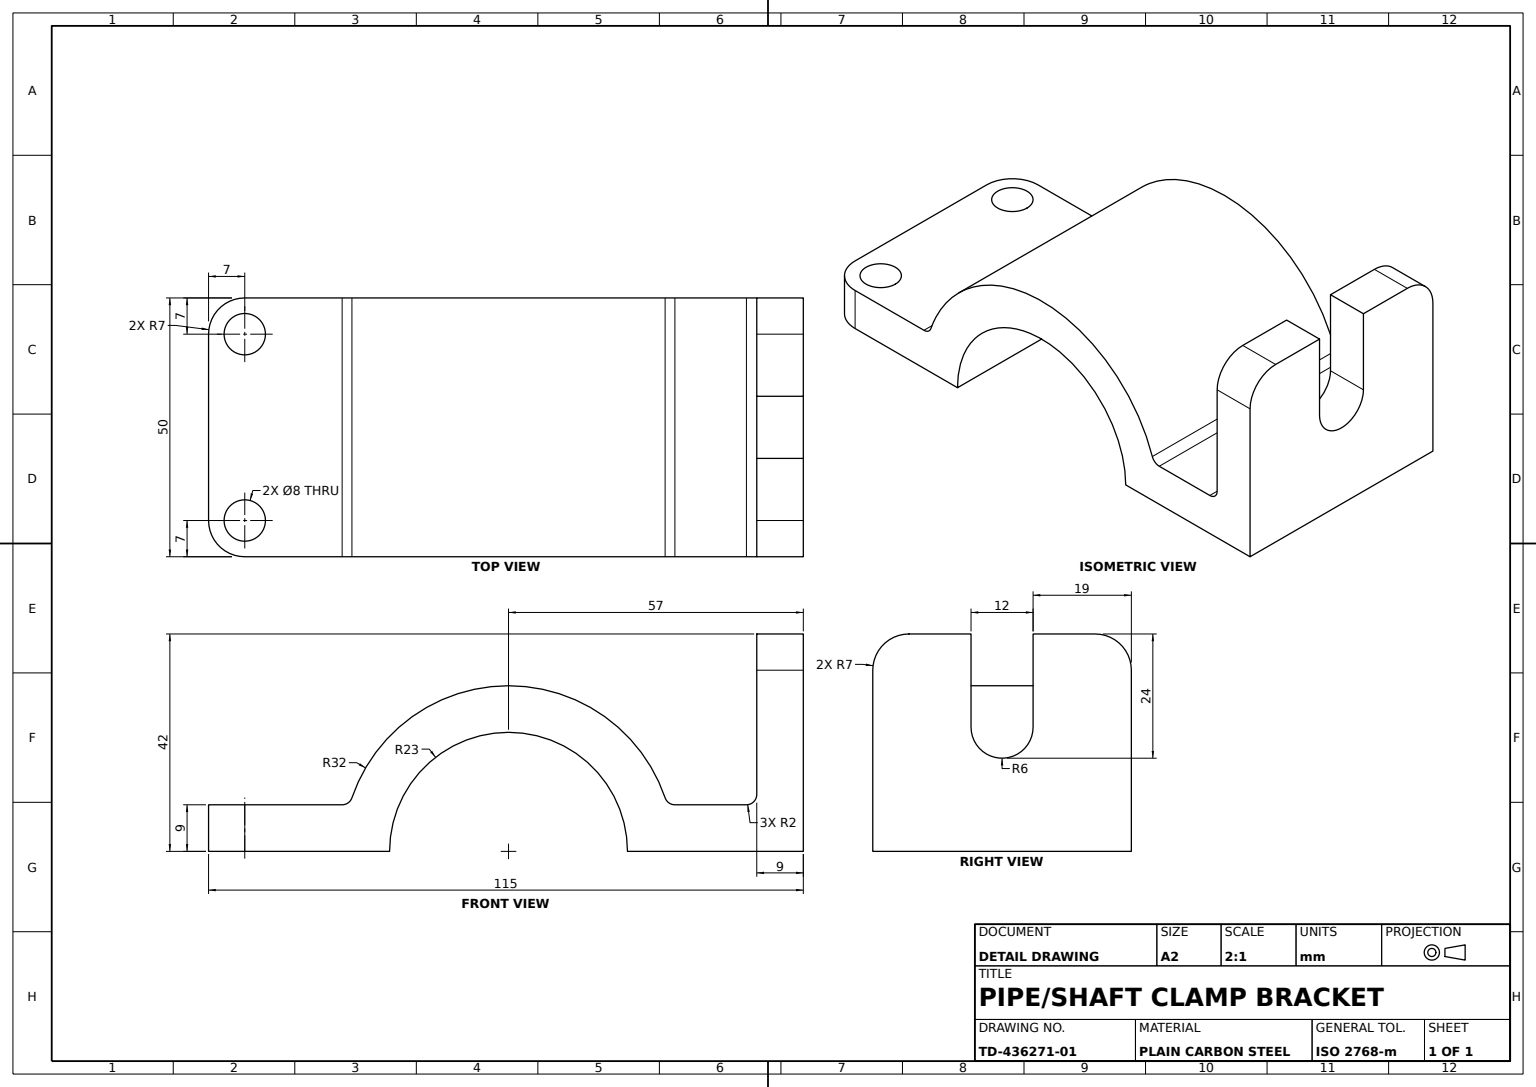
SolidWorks part; units mm, degrees
material "Plain Carbon Steel"
ref_plane "Front Plane" through (0, 0, 0) normal (0, 0, 1) x (1, 0, 0)
ref_plane "Top Plane" through (0, 0, 0) normal (0, 1, 0) x (1, 0, 0)
ref_plane "Right Plane" through (0, 0, 0) normal (1, 0, 0) x (0, 0, -1)
sketch "Saddle Profile Sketch" plane through (0, 0, 0) normal (0, 0, 1) x (1, 0, 0)
  line L0 (-58, 0) -> (-23, 0)
  line L1 (57, 0) -> (57, 42)
  line L2 (57, 42) -> (48, 42)
  line L3 (48, 42) -> (48, 9)
  line L4 (48, 9) -> (30.7083, 9)
  line L5 (-58, 9) -> (-58, 0)
  line L6 (-30.7083, 9) -> (-58, 9)
  line L7 (23, 0) -> (57, 0)
  arc A0 (23, 0) -> (-23, 0) centre (0, 0) ccw
  arc A1 (30.7083, 9) -> (-30.7083, 9) centre (0, 0) ccw
  dimension "D1" = 46
  dimension "D7" = 9
  dimension "D2" = 57
  dimension "D3" = 42
  dimension "D4" = 115
  dimension "D5" = 9
  dimension "D6" = 9
extrude "Saddle Body" add sketch "Saddle Profile Sketch" along normal mid plane 50
fillet "Edge Fillets R2" radius 2 3 edges at (48, 9, 0) (30.7083, 9, 0) (-30.7083, 9, 0)
fillet "Corner Fillets R7" radius 7 4 edges at (52.5, 42, 25) (52.5, 42, -25) (-58, 4.5, -25) (-58, 4.5, 25)
sketch "Flange Holes Sketch" plane through (0, 9, 0) normal (0, 1, 0) x (1, 0, 0)
  circle A0 centre (-51, 18) radius 4
  circle A1 centre (-51, -18) radius 4
  dimension "D1" = 8
  dimension "D2" = 8
extrude "Flange Holes" cut sketch "Flange Holes Sketch" against normal blind 50
sketch "U-Slot Sketch" plane through (57, 0, 0) normal (1, 0, 0) x (0, 0, -1)
  line L0 (0, 24) -> (0, 44.9351) construction
  line L1 (-6, 24) -> (-6, 44.9351)
  line L2 (6, 24) -> (6, 44.9351)
  line L3 (-18, 42) -> (18, 42) construction
  arc A0 (-6, 24) -> (6, 24) centre (0, 24) ccw
  arc A1 (6, 44.9351) -> (-6, 44.9351) centre (0, 44.9351) ccw
  point P3 (0, 34.4676)
  dimension "D1" = 18
  dimension "D2" = 12
  dimension "D3" = 2.9351
extrude "U-Slot Cut" cut sketch "U-Slot Sketch" against normal blind 20
